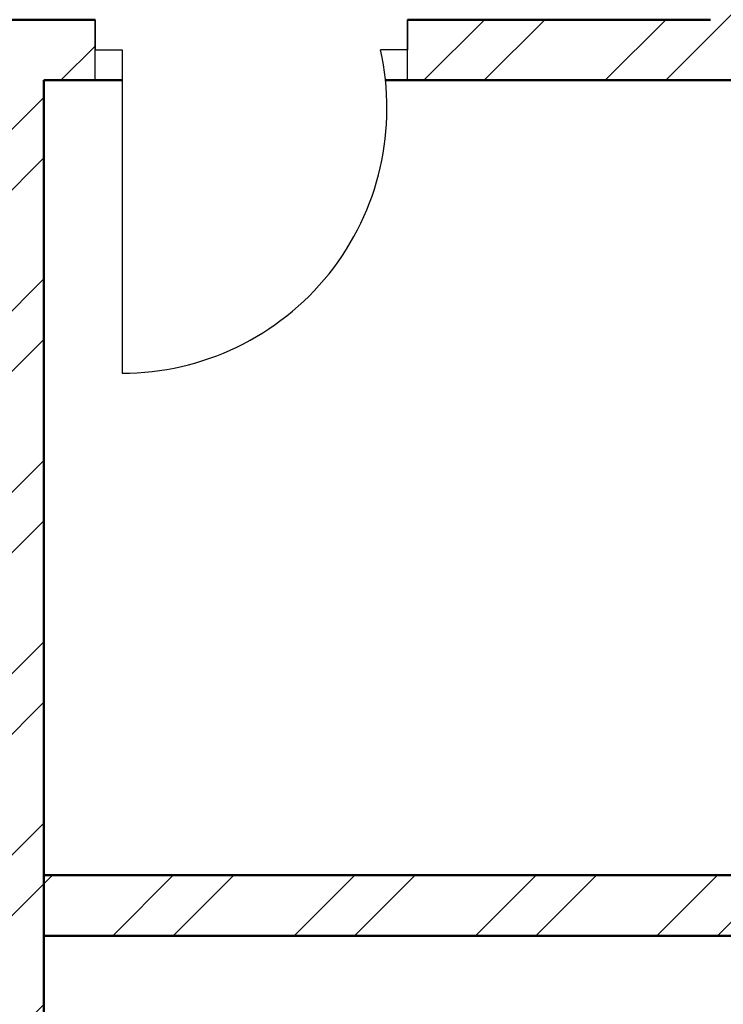
# Model space of a CAD drawing. Units: inches. Extents: x 963 to 2075, y 289 to 2657.
# Tile 32 of 98: x 1594 to 1646, y 1474 to 1547. Entities that reach past the tile are written whole.
import ezdxf

# ---------------------------------------------------------------- set-up
doc = ezdxf.new("R2010")
doc.units = ezdxf.units.IN
for name, color, linetype, lineweight in [('A-DOOR', 4, 'Continuous', 25), ('A-WALL', 7, 'Continuous', 50), ('A-WALL-PATT', 8, 'Continuous', 13)]:
    doc.layers.add(name, color=color, linetype=linetype, lineweight=lineweight)

msp = doc.modelspace()

# ---------------------------------------------------------------- hatches: boundary and pattern name
at = {"layer": 'A-WALL-PATT'}
h = msp.add_hatch(dxfattribs=at)
h.set_pattern_fill('ANSI32', color=256)
h.paths.add_polyline_path([(1910.422, 1929.422), (1910.422, 1963.511), (1905.922, 1963.511), (1905.922, 1929.422), (1845.922, 1929.422), (1845.922, 1993.365), (1843.672, 1993.365), (1841.422, 1993.365), (1841.422, 1951.163), (1841.422, 1924.922), (1853.422, 1924.922), (1853.422, 1913.074), (1857.922, 1913.074), (1857.922, 1924.922), (1910.422, 1924.922)])
h.paths.add_polyline_path([(1857.922, 1853.074), (1853.422, 1853.074), (1853.422, 1826.318), (1841.422, 1826.318), (1674.482, 1826.318), (1674.482, 1821.818), (1853.422, 1821.818), (1857.922, 1821.818)])
h.paths.add_polyline_path([(1857.922, 1821.818), (1853.422, 1821.818), (1853.422, 1807.793), (1857.922, 1807.793)])
h.paths.add_polyline_path([(1857.922, 1747.793), (1853.422, 1747.793), (1853.422, 1713.818), (1809.343, 1713.818), (1809.343, 1709.318), (1905.922, 1709.318), (1905.922, 1688.318), (1910.422, 1688.318), (1910.422, 1713.818), (1857.922, 1713.818)])
h.paths.add_polyline_path([(1830.922, 1542.818), (1837.429, 1542.818), (1837.429, 1545.068), (1837.429, 1547.318), (1823.419, 1547.318), (1823.419, 1545.068), (1823.419, 1542.818), (1826.422, 1542.818), (1826.422, 1482.818), (1742.422, 1482.818), (1742.422, 1505.389), (1737.922, 1505.389), (1737.922, 1478.318), (1830.922, 1478.318)])
h.paths.add_polyline_path([(1938.922, 1619.318), (1934.422, 1619.318), (1910.422, 1619.318), (1910.422, 1628.318), (1908.172, 1628.318), (1905.922, 1628.318), (1905.922, 1614.818), (1934.422, 1614.818), (1934.422, 1547.318), (1905.922, 1547.318), (1899.589, 1547.318), (1899.589, 1542.818), (1910.422, 1542.818), (1938.922, 1542.818)])
h.paths.add_polyline_path([(1803.676, 1547.318), (1773.922, 1547.318), (1773.922, 1709.318), (1777.757, 1709.318), (1777.757, 1713.818), (1701.922, 1713.818), (1701.922, 1697.802), (1706.422, 1697.802), (1706.422, 1709.318), (1769.422, 1709.318), (1769.422, 1662.818), (1706.422, 1662.818), (1706.422, 1674.385), (1701.922, 1674.385), (1701.922, 1662.818), (1675.672, 1662.818), (1675.672, 1658.318), (1769.422, 1658.318), (1769.422, 1547.318), (1729.17, 1547.318), (1729.17, 1542.818), (1737.922, 1542.818), (1737.922, 1529.389), (1742.422, 1529.389), (1742.422, 1542.818), (1803.676, 1542.818)])
h.paths.add_polyline_path([(1595.422, 1542.818), (1599.245, 1542.818), (1599.245, 1547.318), (1584.36, 1547.318), (1584.36, 1542.818), (1590.922, 1542.818), (1590.922, 1436.318), (1595.422, 1436.318), (1595.422, 1440.818)])
h.paths.add_polyline_path([(1693.17, 1547.318), (1649.422, 1547.318), (1649.422, 1658.318), (1652.098, 1658.318), (1652.098, 1660.568), (1652.098, 1662.818), (1649.422, 1662.818), (1649.422, 1680.937), (1647.172, 1680.937), (1644.922, 1680.937), (1644.922, 1547.318), (1622.422, 1547.318), (1622.422, 1545.068), (1622.422, 1542.818), (1649.422, 1542.818), (1679.422, 1542.818), (1679.422, 1529.845), (1681.672, 1529.845), (1683.922, 1529.845), (1683.922, 1542.818), (1693.17, 1542.818), (1693.17, 1545.068)])
h.paths.add_polyline_path([(1683.922, 1505.845), (1679.422, 1505.845), (1679.422, 1483.805), (1595.422, 1483.805), (1595.422, 1479.305), (1683.922, 1479.305)])
h.paths.add_polyline_path([(1402.993, 1547.318), (1376.422, 1547.318), (1376.422, 1675.888), (1374.172, 1675.888), (1371.922, 1675.888), (1371.922, 1662.818), (1368.876, 1662.818), (1368.876, 1658.318), (1371.922, 1658.318), (1371.922, 1547.318), (1335.464, 1547.318), (1335.464, 1542.818), (1337.422, 1542.818), (1337.422, 1526.732), (1341.922, 1526.732), (1341.922, 1542.818), (1371.922, 1542.818), (1402.993, 1542.818)])

# ---------------------------------------------------------------- linework, layer by layer
at = {"layer": 'A-DOOR'}
for p, q in [((1599.245, 1542.818), (1599.245, 1547.318)), ((1599.245, 1547.318), (1599.245, 1545.068)), ((1622.422, 1542.818), (1622.422, 1547.318)), ((1622.422, 1547.318), (1622.422, 1545.068)), ((1599.245, 1545.068), (1601.245, 1545.068)), ((1601.245, 1545.068), (1601.245, 1521.068)), ((1622.422, 1545.068), (1620.422, 1545.068))]:
    msp.add_line(p, q, dxfattribs=at)
msp.add_arc((1601.245, 1540.729), 19.661, 270, 12.7478, dxfattribs=at)
at = {"layer": 'A-WALL'}
for p, q in [((1599.245, 1547.318), (1584.36, 1547.318)), ((1644.922, 1547.318), (1622.422, 1547.318)), ((1595.422, 1542.818), (1595.422, 1440.818)), ((1601.245, 1542.818), (1595.422, 1542.818)), ((1649.422, 1542.818), (1620.795, 1542.818)), ((1679.422, 1483.805), (1595.422, 1483.805)), ((1595.422, 1483.805), (1595.422, 1479.305)), ((1595.422, 1479.305), (1683.922, 1479.305))]:
    msp.add_line(p, q, dxfattribs=at)

doc.saveas('drawing.dxf')
